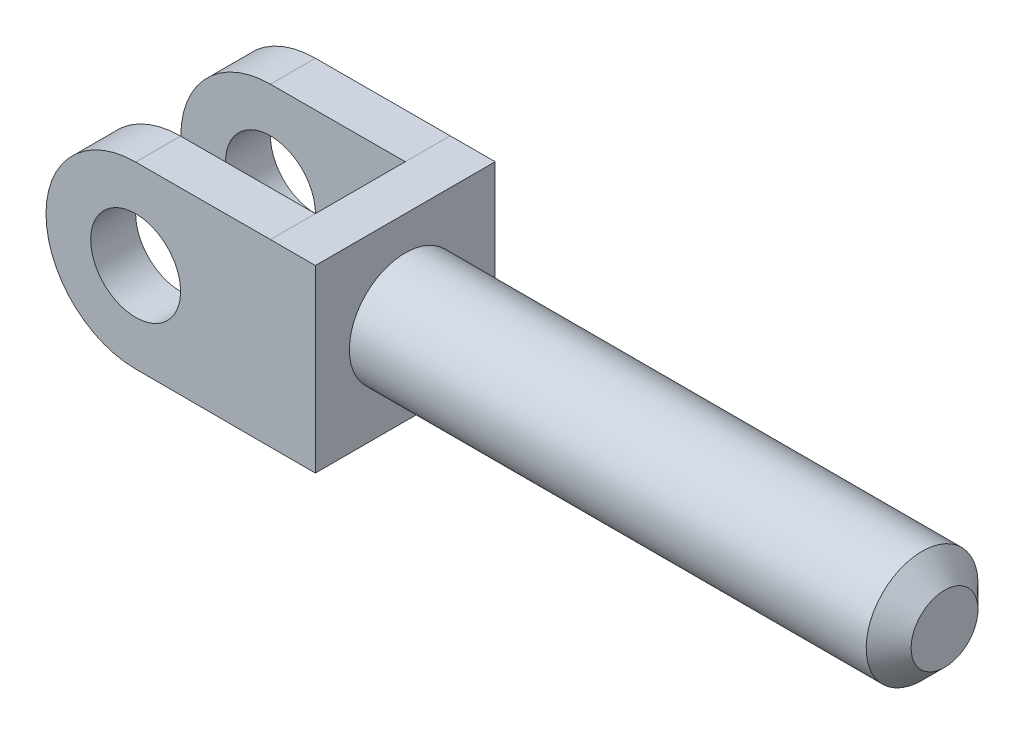
SolidWorks part; units mm, degrees
material "Plain Carbon Steel"
ref_plane "Front Plane" through (0, 0, 0) normal (0, 0, 1) x (1, 0, 0)
ref_plane "Top Plane" through (0, 0, 0) normal (0, 1, 0) x (1, 0, 0)
ref_plane "Right Plane" through (0, 0, 0) normal (1, 0, 0) x (0, 0, -1)
sketch "Clevis Block Sketch" plane through (0, 0, 0) normal (0, 0, 1) x (1, 0, 0)
  line L1 (0, 6.35) -> (3.175, 6.35)
  line L2 (0, 6.35) -> (0, -6.35)
  line L3 (0, -6.35) -> (3.175, -6.35)
  line L4 (3.175, 6.35) -> (3.175, -6.35)
  dimension "D1" = 3.175
  dimension "D2" = 6.35
  dimension "D3" = 12.7
extrude "Clevis Block" add sketch "Clevis Block Sketch" along normal mid plane 12.7
sketch "Shank Sketch Ø7.95" plane through (3.175, 0, 0) normal (1, 0, 0) x (0, 0, -1)
  circle A0 centre (0, 0) radius 3.95
  dimension "D1" = 7.9
extrude "Shank Ø7.95" add sketch "Shank Sketch Ø7.95" along normal blind 38.1
chamfer "Shank End Chamfer" distance 1.5875 angle 45 1 edges at (41.275, 3.95, 0)
sketch "Clevis Ear Sketch" plane through (0, 0, -6.35) normal (0, 0, -1) x (-1, 0, 0)
  line L0 (0, 0) -> (28.3698, 0) construction
  line L1 (-3.175, -6.35) -> (-3.175, 6.35) construction
  line L2 (9.525, 6.3323) -> (0, 6.35)
  line L3 (9.525, -6.3323) -> (0, -6.35)
  line L4 (0, 6.35) -> (0, -6.35)
  circle A0 centre (9.525, 0) radius 3.175
  arc A1 (9.525, -6.3323) -> (9.525, 6.3323) centre (9.525, 0) ccw
  dimension "D1" = 6.35
  dimension "D2" = 12.6647
  dimension "D3" = 12.7
extrude "Clevis Ear" add sketch "Clevis Ear Sketch" against normal blind 3.175
mirror "Clevis Ear Mirror" about plane through (0, 0, 0) normal (0, 0, 1) of "Clevis Ear"
